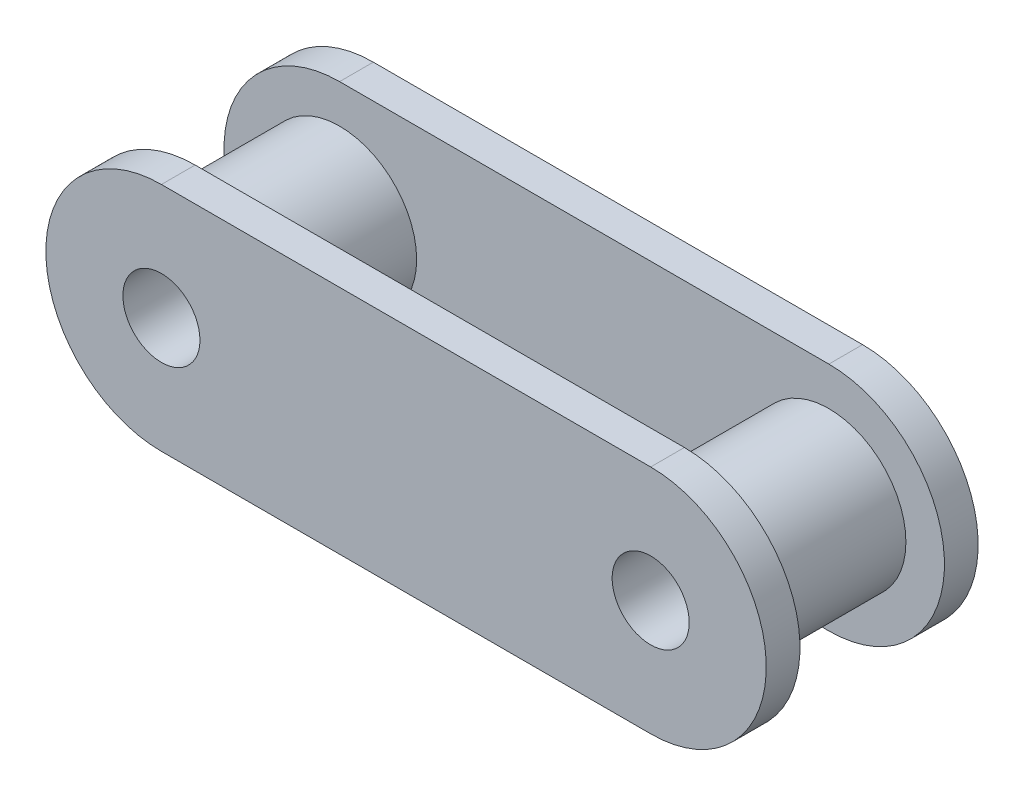
ISO-10303-21;
HEADER;
FILE_DESCRIPTION(('STEP AP214'),'2;1');
FILE_NAME('part.step','',(''),(''),'','','');
FILE_SCHEMA(('AUTOMOTIVE_DESIGN { 1 0 10303 214 1 1 1 1 }'));
ENDSEC;
DATA;
#1=APPLICATION_CONTEXT('core data for automotive mechanical design processes');
#2=APPLICATION_PROTOCOL_DEFINITION('international standard','automotive_design',2000,#1);
#3=PRODUCT_CONTEXT('',#1,'mechanical');
#4=PRODUCT('Part','Part','',(#3));
#5=PRODUCT_RELATED_PRODUCT_CATEGORY('part','',(#4));
#6=PRODUCT_DEFINITION_FORMATION('','',#4);
#7=PRODUCT_DEFINITION_CONTEXT('part definition',#1,'design');
#8=PRODUCT_DEFINITION('design','',#6,#7);
#9=PRODUCT_DEFINITION_SHAPE('','',#8);
#10=(LENGTH_UNIT() NAMED_UNIT(*) SI_UNIT(.MILLI.,.METRE.));
#11=(NAMED_UNIT(*) PLANE_ANGLE_UNIT() SI_UNIT($,.RADIAN.));
#12=(NAMED_UNIT(*) SI_UNIT($,.STERADIAN.) SOLID_ANGLE_UNIT());
#13=UNCERTAINTY_MEASURE_WITH_UNIT(LENGTH_MEASURE(1.E-05),#10,'distance_accuracy_value','');
#14=(GEOMETRIC_REPRESENTATION_CONTEXT(3) GLOBAL_UNCERTAINTY_ASSIGNED_CONTEXT((#13)) GLOBAL_UNIT_ASSIGNED_CONTEXT((#10,
#11,#12)) REPRESENTATION_CONTEXT('',''));
#15=CARTESIAN_POINT('',(0.,0.,0.));
#16=DIRECTION('',(0.,0.,1.));
#17=DIRECTION('',(1.,0.,0.));
#18=AXIS2_PLACEMENT_3D('',#15,#16,#17);
#19=CARTESIAN_POINT('',(0.,0.,3.5));
#20=DIRECTION('',(0.,0.,-1.));
#21=DIRECTION('',(-1.,0.,0.));
#22=AXIS2_PLACEMENT_3D('',#19,#20,#21);
#23=CYLINDRICAL_SURFACE('',#22,12.);
#24=CARTESIAN_POINT('',(0.,0.,0.));
#25=DIRECTION('',(0.,0.,1.));
#26=DIRECTION('',(1.,0.,0.));
#27=AXIS2_PLACEMENT_3D('',#24,#25,#26);
#28=CIRCLE('',#27,12.);
#29=CARTESIAN_POINT('',(0.,12.,0.));
#30=VERTEX_POINT('',#29);
#31=CARTESIAN_POINT('',(0.,-12.,0.));
#32=VERTEX_POINT('',#31);
#33=EDGE_CURVE('E157',#30,#32,#28,.T.);
#34=ORIENTED_EDGE('',*,*,#33,.T.);
#35=DIRECTION('',(0.,0.,-1.));
#36=VECTOR('',#35,1.);
#37=CARTESIAN_POINT('',(0.,-12.,3.5));
#38=LINE('',#37,#36);
#39=CARTESIAN_POINT('',(0.,-12.,3.5));
#40=VERTEX_POINT('',#39);
#41=EDGE_CURVE('E11',#40,#32,#38,.T.);
#42=ORIENTED_EDGE('',*,*,#41,.F.);
#43=CARTESIAN_POINT('',(0.,0.,3.5));
#44=DIRECTION('',(0.,0.,1.));
#45=DIRECTION('',(1.,0.,0.));
#46=AXIS2_PLACEMENT_3D('',#43,#44,#45);
#47=CIRCLE('',#46,12.);
#48=CARTESIAN_POINT('',(0.,12.,3.5));
#49=VERTEX_POINT('',#48);
#50=EDGE_CURVE('E165',#49,#40,#47,.T.);
#51=ORIENTED_EDGE('',*,*,#50,.F.);
#52=DIRECTION('',(0.,0.,-1.));
#53=VECTOR('',#52,1.);
#54=CARTESIAN_POINT('',(0.,12.,3.5));
#55=LINE('',#54,#53);
#56=EDGE_CURVE('E169',#49,#30,#55,.T.);
#57=ORIENTED_EDGE('',*,*,#56,.T.);
#58=EDGE_LOOP('',(#34,#42,#51,#57));
#59=FACE_BOUND('',#58,.T.);
#60=ADVANCED_FACE('F44',(#59),#23,.T.);
#61=CARTESIAN_POINT('',(50.8,-12.,3.5));
#62=DIRECTION('',(0.,1.,0.));
#63=DIRECTION('',(-1.,0.,0.));
#64=AXIS2_PLACEMENT_3D('',#61,#62,#63);
#65=PLANE('',#64);
#66=DIRECTION('',(1.,0.,0.));
#67=VECTOR('',#66,1.);
#68=CARTESIAN_POINT('',(50.8,-12.,0.));
#69=LINE('',#68,#67);
#70=CARTESIAN_POINT('',(50.8,-12.,0.));
#71=VERTEX_POINT('',#70);
#72=EDGE_CURVE('E173',#32,#71,#69,.T.);
#73=ORIENTED_EDGE('',*,*,#72,.T.);
#74=DIRECTION('',(0.,0.,-1.));
#75=VECTOR('',#74,1.);
#76=CARTESIAN_POINT('',(50.8,-12.,3.5));
#77=LINE('',#76,#75);
#78=CARTESIAN_POINT('',(50.8,-12.,3.5));
#79=VERTEX_POINT('',#78);
#80=EDGE_CURVE('E52',#79,#71,#77,.T.);
#81=ORIENTED_EDGE('',*,*,#80,.F.);
#82=DIRECTION('',(1.,0.,0.));
#83=VECTOR('',#82,1.);
#84=CARTESIAN_POINT('',(50.8,-12.,3.5));
#85=LINE('',#84,#83);
#86=EDGE_CURVE('E95',#40,#79,#85,.T.);
#87=ORIENTED_EDGE('',*,*,#86,.F.);
#88=ORIENTED_EDGE('',*,*,#41,.T.);
#89=EDGE_LOOP('',(#73,#81,#87,#88));
#90=FACE_BOUND('',#89,.T.);
#91=ADVANCED_FACE('F198',(#90),#65,.F.);
#92=CARTESIAN_POINT('',(50.8,0.,3.5));
#93=DIRECTION('',(0.,0.,-1.));
#94=DIRECTION('',(-1.,0.,0.));
#95=AXIS2_PLACEMENT_3D('',#92,#93,#94);
#96=CYLINDRICAL_SURFACE('',#95,12.);
#97=CARTESIAN_POINT('',(50.8,0.,0.));
#98=DIRECTION('',(0.,0.,1.));
#99=DIRECTION('',(1.,0.,0.));
#100=AXIS2_PLACEMENT_3D('',#97,#98,#99);
#101=CIRCLE('',#100,12.);
#102=CARTESIAN_POINT('',(50.8,12.,0.));
#103=VERTEX_POINT('',#102);
#104=EDGE_CURVE('E80',#71,#103,#101,.T.);
#105=ORIENTED_EDGE('',*,*,#104,.T.);
#106=DIRECTION('',(0.,0.,-1.));
#107=VECTOR('',#106,1.);
#108=CARTESIAN_POINT('',(50.8,12.,3.5));
#109=LINE('',#108,#107);
#110=CARTESIAN_POINT('',(50.8,12.,3.5));
#111=VERTEX_POINT('',#110);
#112=EDGE_CURVE('E177',#111,#103,#109,.T.);
#113=ORIENTED_EDGE('',*,*,#112,.F.);
#114=CARTESIAN_POINT('',(50.8,0.,3.5));
#115=DIRECTION('',(0.,0.,1.));
#116=DIRECTION('',(1.,0.,0.));
#117=AXIS2_PLACEMENT_3D('',#114,#115,#116);
#118=CIRCLE('',#117,12.);
#119=EDGE_CURVE('E164',#79,#111,#118,.T.);
#120=ORIENTED_EDGE('',*,*,#119,.F.);
#121=ORIENTED_EDGE('',*,*,#80,.T.);
#122=EDGE_LOOP('',(#105,#113,#120,#121));
#123=FACE_BOUND('',#122,.T.);
#124=ADVANCED_FACE('F178',(#123),#96,.T.);
#125=CARTESIAN_POINT('',(0.,12.,3.5));
#126=DIRECTION('',(0.,-1.,0.));
#127=DIRECTION('',(1.,0.,0.));
#128=AXIS2_PLACEMENT_3D('',#125,#126,#127);
#129=PLANE('',#128);
#130=DIRECTION('',(-1.,0.,0.));
#131=VECTOR('',#130,1.);
#132=CARTESIAN_POINT('',(0.,12.,0.));
#133=LINE('',#132,#131);
#134=EDGE_CURVE('E81',#103,#30,#133,.T.);
#135=ORIENTED_EDGE('',*,*,#134,.T.);
#136=ORIENTED_EDGE('',*,*,#56,.F.);
#137=DIRECTION('',(-1.,0.,0.));
#138=VECTOR('',#137,1.);
#139=CARTESIAN_POINT('',(0.,12.,3.5));
#140=LINE('',#139,#138);
#141=EDGE_CURVE('E63',#111,#49,#140,.T.);
#142=ORIENTED_EDGE('',*,*,#141,.F.);
#143=ORIENTED_EDGE('',*,*,#112,.T.);
#144=EDGE_LOOP('',(#135,#136,#142,#143));
#145=FACE_BOUND('',#144,.T.);
#146=ADVANCED_FACE('F183',(#145),#129,.F.);
#147=CARTESIAN_POINT('',(0.,0.,3.5));
#148=DIRECTION('',(0.,0.,1.));
#149=DIRECTION('',(1.,0.,0.));
#150=AXIS2_PLACEMENT_3D('',#147,#148,#149);
#151=PLANE('',#150);
#152=CARTESIAN_POINT('',(50.8,0.,3.5));
#153=DIRECTION('',(0.,0.,1.));
#154=DIRECTION('',(1.,0.,0.));
#155=AXIS2_PLACEMENT_3D('',#152,#153,#154);
#156=CIRCLE('',#155,8.);
#157=CARTESIAN_POINT('',(58.8,0.,3.5));
#158=VERTEX_POINT('',#157);
#159=EDGE_CURVE('E145',#158,#158,#156,.T.);
#160=ORIENTED_EDGE('',*,*,#159,.F.);
#161=EDGE_LOOP('',(#160));
#162=FACE_BOUND('',#161,.T.);
#163=CARTESIAN_POINT('',(0.,0.,3.5));
#164=DIRECTION('',(0.,0.,1.));
#165=DIRECTION('',(1.,0.,0.));
#166=AXIS2_PLACEMENT_3D('',#163,#164,#165);
#167=CIRCLE('',#166,8.);
#168=CARTESIAN_POINT('',(8.,0.,3.5));
#169=VERTEX_POINT('',#168);
#170=EDGE_CURVE('E152',#169,#169,#167,.T.);
#171=ORIENTED_EDGE('',*,*,#170,.F.);
#172=EDGE_LOOP('',(#171));
#173=FACE_BOUND('',#172,.T.);
#174=ORIENTED_EDGE('',*,*,#50,.T.);
#175=ORIENTED_EDGE('',*,*,#86,.T.);
#176=ORIENTED_EDGE('',*,*,#119,.T.);
#177=ORIENTED_EDGE('',*,*,#141,.T.);
#178=EDGE_LOOP('',(#174,#175,#176,#177));
#179=FACE_BOUND('',#178,.T.);
#180=ADVANCED_FACE('F189',(#162,#173,#179),#151,.T.);
#181=CARTESIAN_POINT('',(0.,0.,0.));
#182=DIRECTION('',(0.,0.,1.));
#183=DIRECTION('',(1.,0.,0.));
#184=AXIS2_PLACEMENT_3D('',#181,#182,#183);
#185=PLANE('',#184);
#186=CARTESIAN_POINT('',(0.,0.,0.));
#187=DIRECTION('',(0.,0.,1.));
#188=DIRECTION('',(1.,0.,0.));
#189=AXIS2_PLACEMENT_3D('',#186,#187,#188);
#190=CIRCLE('',#189,4.);
#191=CARTESIAN_POINT('',(4.,0.,0.));
#192=VERTEX_POINT('',#191);
#193=EDGE_CURVE('E373',#192,#192,#190,.T.);
#194=ORIENTED_EDGE('',*,*,#193,.T.);
#195=EDGE_LOOP('',(#194));
#196=FACE_BOUND('',#195,.T.);
#197=CARTESIAN_POINT('',(50.8,0.,0.));
#198=DIRECTION('',(0.,0.,1.));
#199=DIRECTION('',(1.,0.,0.));
#200=AXIS2_PLACEMENT_3D('',#197,#198,#199);
#201=CIRCLE('',#200,4.);
#202=CARTESIAN_POINT('',(54.8,0.,0.));
#203=VERTEX_POINT('',#202);
#204=EDGE_CURVE('E380',#203,#203,#201,.T.);
#205=ORIENTED_EDGE('',*,*,#204,.T.);
#206=EDGE_LOOP('',(#205));
#207=FACE_BOUND('',#206,.T.);
#208=ORIENTED_EDGE('',*,*,#33,.F.);
#209=ORIENTED_EDGE('',*,*,#134,.F.);
#210=ORIENTED_EDGE('',*,*,#104,.F.);
#211=ORIENTED_EDGE('',*,*,#72,.F.);
#212=EDGE_LOOP('',(#208,#209,#210,#211));
#213=FACE_BOUND('',#212,.T.);
#214=ADVANCED_FACE('F182',(#196,#207,#213),#185,.F.);
#215=CARTESIAN_POINT('',(0.,0.,18.5));
#216=DIRECTION('',(0.,0.,-1.));
#217=DIRECTION('',(-1.,0.,0.));
#218=AXIS2_PLACEMENT_3D('',#215,#216,#217);
#219=CYLINDRICAL_SURFACE('',#218,8.);
#220=CARTESIAN_POINT('',(0.,0.,18.5));
#221=DIRECTION('',(0.,0.,1.));
#222=DIRECTION('',(1.,0.,0.));
#223=AXIS2_PLACEMENT_3D('',#220,#221,#222);
#224=CIRCLE('',#223,8.);
#225=CARTESIAN_POINT('',(8.,0.,18.5));
#226=VERTEX_POINT('',#225);
#227=EDGE_CURVE('E156',#226,#226,#224,.T.);
#228=ORIENTED_EDGE('',*,*,#227,.F.);
#229=EDGE_LOOP('',(#228));
#230=FACE_BOUND('',#229,.T.);
#231=ORIENTED_EDGE('',*,*,#170,.T.);
#232=EDGE_LOOP('',(#231));
#233=FACE_BOUND('',#232,.T.);
#234=ADVANCED_FACE('F235',(#230,#233),#219,.T.);
#235=CARTESIAN_POINT('',(50.8,0.,18.5));
#236=DIRECTION('',(0.,0.,-1.));
#237=DIRECTION('',(-1.,0.,0.));
#238=AXIS2_PLACEMENT_3D('',#235,#236,#237);
#239=CYLINDRICAL_SURFACE('',#238,8.);
#240=CARTESIAN_POINT('',(50.8,0.,18.5));
#241=DIRECTION('',(0.,0.,1.));
#242=DIRECTION('',(1.,0.,0.));
#243=AXIS2_PLACEMENT_3D('',#240,#241,#242);
#244=CIRCLE('',#243,8.);
#245=CARTESIAN_POINT('',(58.8,0.,18.5));
#246=VERTEX_POINT('',#245);
#247=EDGE_CURVE('E150',#246,#246,#244,.T.);
#248=ORIENTED_EDGE('',*,*,#247,.F.);
#249=EDGE_LOOP('',(#248));
#250=FACE_BOUND('',#249,.T.);
#251=ORIENTED_EDGE('',*,*,#159,.T.);
#252=EDGE_LOOP('',(#251));
#253=FACE_BOUND('',#252,.T.);
#254=ADVANCED_FACE('F242',(#250,#253),#239,.T.);
#255=CARTESIAN_POINT('',(0.,0.,22.));
#256=DIRECTION('',(0.,0.,-1.));
#257=DIRECTION('',(-1.,0.,0.));
#258=AXIS2_PLACEMENT_3D('',#255,#256,#257);
#259=CYLINDRICAL_SURFACE('',#258,12.);
#260=CARTESIAN_POINT('',(0.,0.,18.5));
#261=DIRECTION('',(0.,0.,1.));
#262=DIRECTION('',(1.,0.,0.));
#263=AXIS2_PLACEMENT_3D('',#260,#261,#262);
#264=CIRCLE('',#263,12.);
#265=CARTESIAN_POINT('',(0.,12.,18.5));
#266=VERTEX_POINT('',#265);
#267=CARTESIAN_POINT('',(0.,-12.,18.5));
#268=VERTEX_POINT('',#267);
#269=EDGE_CURVE('E141',#266,#268,#264,.T.);
#270=ORIENTED_EDGE('',*,*,#269,.T.);
#271=DIRECTION('',(0.,0.,-1.));
#272=VECTOR('',#271,1.);
#273=CARTESIAN_POINT('',(0.,-12.,22.));
#274=LINE('',#273,#272);
#275=CARTESIAN_POINT('',(0.,-12.,22.));
#276=VERTEX_POINT('',#275);
#277=EDGE_CURVE('E123',#276,#268,#274,.T.);
#278=ORIENTED_EDGE('',*,*,#277,.F.);
#279=CARTESIAN_POINT('',(0.,0.,22.));
#280=DIRECTION('',(0.,0.,1.));
#281=DIRECTION('',(1.,0.,0.));
#282=AXIS2_PLACEMENT_3D('',#279,#280,#281);
#283=CIRCLE('',#282,12.);
#284=CARTESIAN_POINT('',(0.,12.,22.));
#285=VERTEX_POINT('',#284);
#286=EDGE_CURVE('E128',#285,#276,#283,.T.);
#287=ORIENTED_EDGE('',*,*,#286,.F.);
#288=DIRECTION('',(0.,0.,-1.));
#289=VECTOR('',#288,1.);
#290=CARTESIAN_POINT('',(0.,12.,22.));
#291=LINE('',#290,#289);
#292=EDGE_CURVE('E389',#285,#266,#291,.T.);
#293=ORIENTED_EDGE('',*,*,#292,.T.);
#294=EDGE_LOOP('',(#270,#278,#287,#293));
#295=FACE_BOUND('',#294,.T.);
#296=ADVANCED_FACE('F143',(#295),#259,.T.);
#297=CARTESIAN_POINT('',(50.8,-12.,22.));
#298=DIRECTION('',(0.,1.,0.));
#299=DIRECTION('',(-1.,0.,0.));
#300=AXIS2_PLACEMENT_3D('',#297,#298,#299);
#301=PLANE('',#300);
#302=DIRECTION('',(1.,0.,0.));
#303=VECTOR('',#302,1.);
#304=CARTESIAN_POINT('',(50.8,-12.,18.5));
#305=LINE('',#304,#303);
#306=CARTESIAN_POINT('',(50.8,-12.,18.5));
#307=VERTEX_POINT('',#306);
#308=EDGE_CURVE('E388',#268,#307,#305,.T.);
#309=ORIENTED_EDGE('',*,*,#308,.T.);
#310=DIRECTION('',(0.,0.,-1.));
#311=VECTOR('',#310,1.);
#312=CARTESIAN_POINT('',(50.8,-12.,22.));
#313=LINE('',#312,#311);
#314=CARTESIAN_POINT('',(50.8,-12.,22.));
#315=VERTEX_POINT('',#314);
#316=EDGE_CURVE('E127',#315,#307,#313,.T.);
#317=ORIENTED_EDGE('',*,*,#316,.F.);
#318=DIRECTION('',(1.,0.,0.));
#319=VECTOR('',#318,1.);
#320=CARTESIAN_POINT('',(50.8,-12.,22.));
#321=LINE('',#320,#319);
#322=EDGE_CURVE('E120',#276,#315,#321,.T.);
#323=ORIENTED_EDGE('',*,*,#322,.F.);
#324=ORIENTED_EDGE('',*,*,#277,.T.);
#325=EDGE_LOOP('',(#309,#317,#323,#324));
#326=FACE_BOUND('',#325,.T.);
#327=ADVANCED_FACE('F122',(#326),#301,.F.);
#328=CARTESIAN_POINT('',(50.8,0.,22.));
#329=DIRECTION('',(0.,0.,-1.));
#330=DIRECTION('',(-1.,0.,0.));
#331=AXIS2_PLACEMENT_3D('',#328,#329,#330);
#332=CYLINDRICAL_SURFACE('',#331,12.);
#333=CARTESIAN_POINT('',(50.8,0.,18.5));
#334=DIRECTION('',(0.,0.,1.));
#335=DIRECTION('',(1.,0.,0.));
#336=AXIS2_PLACEMENT_3D('',#333,#334,#335);
#337=CIRCLE('',#336,12.);
#338=CARTESIAN_POINT('',(50.8,12.,18.5));
#339=VERTEX_POINT('',#338);
#340=EDGE_CURVE('E394',#307,#339,#337,.T.);
#341=ORIENTED_EDGE('',*,*,#340,.T.);
#342=DIRECTION('',(0.,0.,-1.));
#343=VECTOR('',#342,1.);
#344=CARTESIAN_POINT('',(50.8,12.,22.));
#345=LINE('',#344,#343);
#346=CARTESIAN_POINT('',(50.8,12.,22.));
#347=VERTEX_POINT('',#346);
#348=EDGE_CURVE('E149',#347,#339,#345,.T.);
#349=ORIENTED_EDGE('',*,*,#348,.F.);
#350=CARTESIAN_POINT('',(50.8,0.,22.));
#351=DIRECTION('',(0.,0.,1.));
#352=DIRECTION('',(1.,0.,0.));
#353=AXIS2_PLACEMENT_3D('',#350,#351,#352);
#354=CIRCLE('',#353,12.);
#355=EDGE_CURVE('E129',#315,#347,#354,.T.);
#356=ORIENTED_EDGE('',*,*,#355,.F.);
#357=ORIENTED_EDGE('',*,*,#316,.T.);
#358=EDGE_LOOP('',(#341,#349,#356,#357));
#359=FACE_BOUND('',#358,.T.);
#360=ADVANCED_FACE('F272',(#359),#332,.T.);
#361=CARTESIAN_POINT('',(0.,12.,22.));
#362=DIRECTION('',(0.,-1.,0.));
#363=DIRECTION('',(1.,0.,0.));
#364=AXIS2_PLACEMENT_3D('',#361,#362,#363);
#365=PLANE('',#364);
#366=DIRECTION('',(-1.,0.,0.));
#367=VECTOR('',#366,1.);
#368=CARTESIAN_POINT('',(0.,12.,18.5));
#369=LINE('',#368,#367);
#370=EDGE_CURVE('E139',#339,#266,#369,.T.);
#371=ORIENTED_EDGE('',*,*,#370,.T.);
#372=ORIENTED_EDGE('',*,*,#292,.F.);
#373=DIRECTION('',(-1.,0.,0.));
#374=VECTOR('',#373,1.);
#375=CARTESIAN_POINT('',(0.,12.,22.));
#376=LINE('',#375,#374);
#377=EDGE_CURVE('E131',#347,#285,#376,.T.);
#378=ORIENTED_EDGE('',*,*,#377,.F.);
#379=ORIENTED_EDGE('',*,*,#348,.T.);
#380=EDGE_LOOP('',(#371,#372,#378,#379));
#381=FACE_BOUND('',#380,.T.);
#382=ADVANCED_FACE('F284',(#381),#365,.F.);
#383=CARTESIAN_POINT('',(0.,0.,22.));
#384=DIRECTION('',(0.,0.,1.));
#385=DIRECTION('',(1.,0.,0.));
#386=AXIS2_PLACEMENT_3D('',#383,#384,#385);
#387=PLANE('',#386);
#388=CARTESIAN_POINT('',(0.,0.,22.));
#389=DIRECTION('',(0.,0.,1.));
#390=DIRECTION('',(1.,0.,0.));
#391=AXIS2_PLACEMENT_3D('',#388,#389,#390);
#392=CIRCLE('',#391,4.);
#393=CARTESIAN_POINT('',(4.,0.,22.));
#394=VERTEX_POINT('',#393);
#395=EDGE_CURVE('E376',#394,#394,#392,.T.);
#396=ORIENTED_EDGE('',*,*,#395,.F.);
#397=EDGE_LOOP('',(#396));
#398=FACE_BOUND('',#397,.T.);
#399=CARTESIAN_POINT('',(50.8,0.,22.));
#400=DIRECTION('',(0.,0.,1.));
#401=DIRECTION('',(1.,0.,0.));
#402=AXIS2_PLACEMENT_3D('',#399,#400,#401);
#403=CIRCLE('',#402,4.);
#404=CARTESIAN_POINT('',(54.8,0.,22.));
#405=VERTEX_POINT('',#404);
#406=EDGE_CURVE('E381',#405,#405,#403,.T.);
#407=ORIENTED_EDGE('',*,*,#406,.F.);
#408=EDGE_LOOP('',(#407));
#409=FACE_BOUND('',#408,.T.);
#410=ORIENTED_EDGE('',*,*,#286,.T.);
#411=ORIENTED_EDGE('',*,*,#322,.T.);
#412=ORIENTED_EDGE('',*,*,#355,.T.);
#413=ORIENTED_EDGE('',*,*,#377,.T.);
#414=EDGE_LOOP('',(#410,#411,#412,#413));
#415=FACE_BOUND('',#414,.T.);
#416=ADVANCED_FACE('F132',(#398,#409,#415),#387,.T.);
#417=CARTESIAN_POINT('',(0.,0.,18.5));
#418=DIRECTION('',(0.,0.,1.));
#419=DIRECTION('',(1.,0.,0.));
#420=AXIS2_PLACEMENT_3D('',#417,#418,#419);
#421=PLANE('',#420);
#422=ORIENTED_EDGE('',*,*,#227,.T.);
#423=EDGE_LOOP('',(#422));
#424=FACE_BOUND('',#423,.T.);
#425=ORIENTED_EDGE('',*,*,#247,.T.);
#426=EDGE_LOOP('',(#425));
#427=FACE_BOUND('',#426,.T.);
#428=ORIENTED_EDGE('',*,*,#269,.F.);
#429=ORIENTED_EDGE('',*,*,#370,.F.);
#430=ORIENTED_EDGE('',*,*,#340,.F.);
#431=ORIENTED_EDGE('',*,*,#308,.F.);
#432=EDGE_LOOP('',(#428,#429,#430,#431));
#433=FACE_BOUND('',#432,.T.);
#434=ADVANCED_FACE('F296',(#424,#427,#433),#421,.F.);
#435=CARTESIAN_POINT('',(50.8,0.,0.));
#436=DIRECTION('',(0.,0.,1.));
#437=DIRECTION('',(1.,0.,0.));
#438=AXIS2_PLACEMENT_3D('',#435,#436,#437);
#439=CYLINDRICAL_SURFACE('',#438,4.);
#440=ORIENTED_EDGE('',*,*,#204,.F.);
#441=EDGE_LOOP('',(#440));
#442=FACE_BOUND('',#441,.T.);
#443=ORIENTED_EDGE('',*,*,#406,.T.);
#444=EDGE_LOOP('',(#443));
#445=FACE_BOUND('',#444,.T.);
#446=ADVANCED_FACE('F313',(#442,#445),#439,.F.);
#447=CARTESIAN_POINT('',(0.,0.,0.));
#448=DIRECTION('',(0.,0.,1.));
#449=DIRECTION('',(1.,0.,0.));
#450=AXIS2_PLACEMENT_3D('',#447,#448,#449);
#451=CYLINDRICAL_SURFACE('',#450,4.);
#452=ORIENTED_EDGE('',*,*,#193,.F.);
#453=EDGE_LOOP('',(#452));
#454=FACE_BOUND('',#453,.T.);
#455=ORIENTED_EDGE('',*,*,#395,.T.);
#456=EDGE_LOOP('',(#455));
#457=FACE_BOUND('',#456,.T.);
#458=ADVANCED_FACE('F325',(#454,#457),#451,.F.);
#459=CLOSED_SHELL('',(#60,#91,#124,#146,#180,#214,#234,#254,#296,#327,#360,#382,#416,#434,#446,#458));
#460=MANIFOLD_SOLID_BREP('B2',#459);
#461=ADVANCED_BREP_SHAPE_REPRESENTATION('',(#18,#460),#14);
#462=SHAPE_DEFINITION_REPRESENTATION(#9,#461);
ENDSEC;
END-ISO-10303-21;
